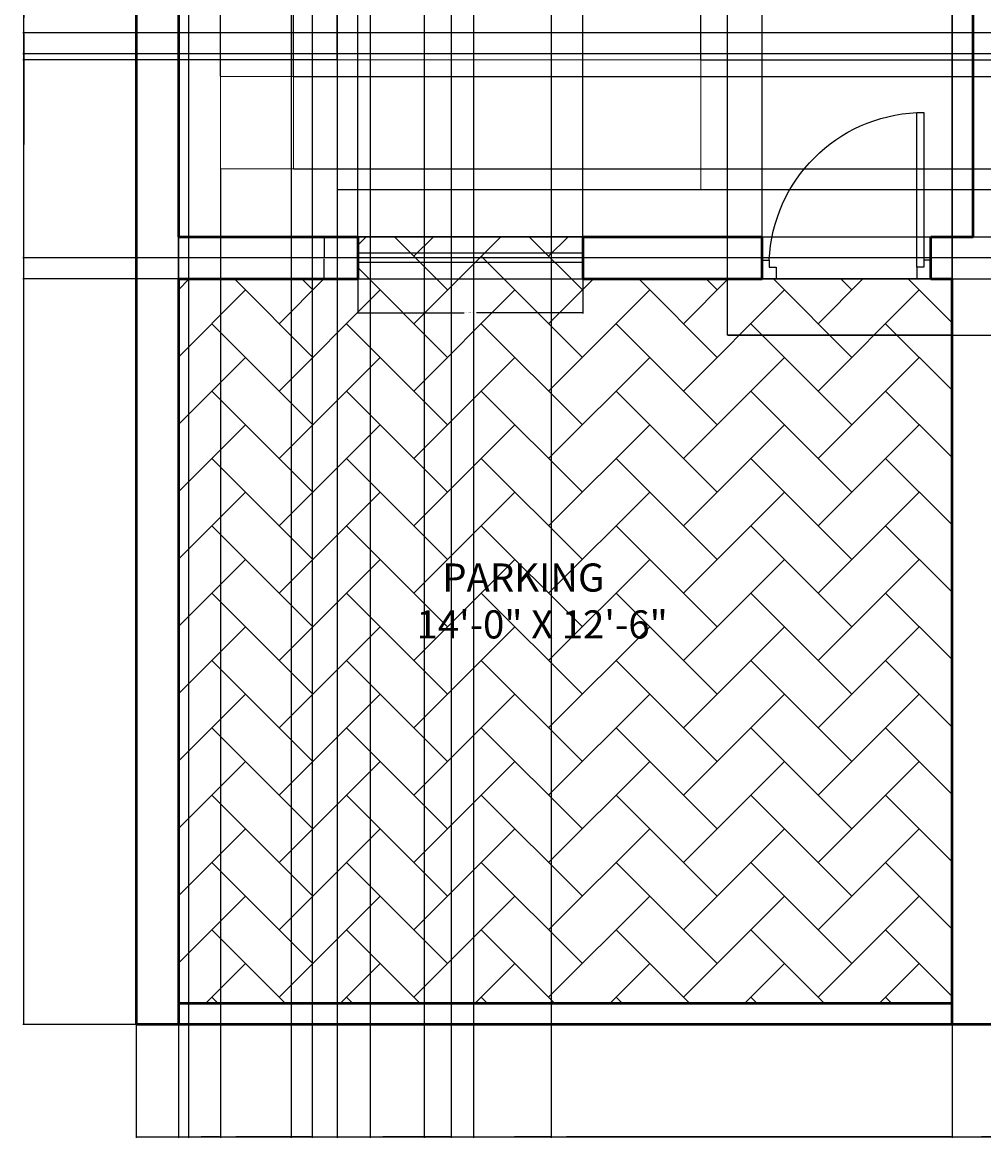
# Model space of a CAD drawing. Units: inches. Extents: x 2330 to 2739, y 947 to 1475.
# Tile 1 of 6: x 2330 to 2535, y 947 to 1185. Entities that reach past the tile are written whole.
import ezdxf

# ---------------------------------------------------------------- set-up
doc = ezdxf.new("R2010")
doc.units = ezdxf.units.IN
for name, color, linetype, lineweight in [('A-ANNO-DIMS', 2, 'Continuous', 18), ('A-AREA-IDEN', 7, 'Continuous', 25), ('A-FLOR-PATT', 252, 'Continuous', 13), ('door', 150, 'Continuous', 25), ('furniture', 9, 'Continuous', 18), ('staircase', 51, 'Continuous', 25), ('wall', 7, 'Continuous', 50), ('window', 40, 'Continuous', 25)]:
    doc.layers.add(name, color=color, linetype=linetype, lineweight=lineweight)
doc.styles.get("Standard").update_dxf_attribs({"font": 'arial.ttf'})
doc.dimstyles.get("Standard").update_dxf_attribs({"dimtxt": 0.18, "dimasz": 0.18, "dimexe": 0.18, "dimexo": 0.0625, "dimgap": 0.09, "dimtad": 0, "dimtih": 1, "dimtoh": 1, "dimdec": 4, "dimzin": 0, "dimdsep": 46, "dimtxsty": 'Standard', "dimcen": 0.09, "dimadec": 0, "dimazin": 0, "dimtfac": 1, "dimtdec": 4, "dimtofl": 0, "dimtmove": 0, "dimatfit": 3, "dimfxl": 1, "dimtolj": 1, "dimtzin": 0, "dimarcsym": 0})

# ---------------------------------------------------------------- blocks, each defined once
blk = doc.blocks.new('w1')
at = {"layer": 'window'}
for p, q in [((2786.57, 1274.71), (2786.57, 1226.71)), ((2788.57, 1274.71), (2788.57, 1226.71))]:
    blk.add_line(p, q, dxfattribs=at)
blk.add_lwpolyline([(2783.07, 1226.71), (2792.07, 1226.71), (2792.07, 1274.71), (2783.07, 1274.71)], close=True, dxfattribs=at)
blk = doc.blocks.new('d1')
at = {"layer": 'door'}
blk.add_line((2897.27, 1313.4), (2933.27, 1313.4), dxfattribs=at)
blk.add_lwpolyline([(2898.77, 1315.9), (2900.27, 1315.9), (2900.27, 1348.9), (2898.77, 1348.9)], close=True, dxfattribs=at)
for points in [[(2900.27, 1313.4), (2897.27, 1313.4), (2897.27, 1317.4), (2898.77, 1317.4), (2898.77, 1315.9), (2900.27, 1315.9), (2900.27, 1313.4)], [(2930.27, 1313.4), (2933.27, 1313.4), (2933.27, 1317.4), (2931.77, 1317.4), (2931.77, 1315.9), (2930.27, 1315.9), (2930.27, 1313.4)]]:
    blk.add_lwpolyline(points, dxfattribs=at)
blk.add_arc((2898.77, 1315.9), 33.03, 2.6026, 87.3974, dxfattribs=at)
blk = doc.blocks.new('*D12')
at = {"layer": 'A-ANNO-DIMS', "color": 0, "lineweight": -2, "transparency": 16777216}
for p, q in [((2401.93, 1130.22), (2401.93, 1122.9)), ((2449.93, 1130.22), (2449.93, 1122.9)), ((2402.11, 1123.08), (2424.59, 1123.08)), ((2449.75, 1123.08), (2427.27, 1123.08))]:
    blk.add_line(p, q, dxfattribs=at)
at = {"layer": 'A-ANNO-DIMS', "color": 0, "transparency": 16777216}
for points in [[(2402.11, 1123.11), (2402.11, 1123.05), (2401.93, 1123.08)], [(2449.75, 1123.11), (2449.75, 1123.05), (2449.93, 1123.08)]]:
    blk.add_solid(points, dxfattribs=at)
at = {"layer": 'Defpoints', "color": 0, "transparency": 16777216}
for p in [(2401.93, 1130.28), (2449.93, 1130.28), (2449.93, 1123.08)]:
    blk.add_point(p, dxfattribs=at)
at = {"layer": 'A-ANNO-DIMS', "color": 0, "transparency": 16777216, "insert": (2425.93, 1123.08), "char_height": 0.18, "attachment_point": 5}
blk.add_mtext('\\A1;WINDOW W1 48 TYP.', dxfattribs=at)
blk = doc.blocks.new('*D13')
at = {"layer": 'A-ANNO-DIMS', "color": 0, "lineweight": -2, "transparency": 16777216}
for p, q in [((2401.87, 1139.28), (2394.55, 1139.28)), ((2394.73, 1139.1), (2394.73, 1134.96)), ((2394.73, 1130.46), (2394.73, 1134.6)), ((2401.87, 1130.28), (2394.55, 1130.28))]:
    blk.add_line(p, q, dxfattribs=at)
at = {"layer": 'A-ANNO-DIMS', "color": 0, "transparency": 16777216}
for points in [[(2394.7, 1139.1), (2394.76, 1139.1), (2394.73, 1139.28)], [(2394.7, 1130.46), (2394.76, 1130.46), (2394.73, 1130.28)]]:
    blk.add_solid(points, dxfattribs=at)
at = {"layer": 'Defpoints', "color": 0, "transparency": 16777216}
for p in [(2401.93, 1139.28), (2394.73, 1130.28), (2401.93, 1130.28)]:
    blk.add_point(p, dxfattribs=at)
at = {"layer": 'A-ANNO-DIMS', "color": 0, "transparency": 16777216, "insert": (2394.73, 1134.78), "char_height": 0.18, "attachment_point": 5}
blk.add_mtext('\\A1;9 TYP.', dxfattribs=at)
blk = doc.blocks.new('*D24')
at = {"layer": 'A-ANNO-DIMS', "color": 0, "lineweight": -2, "transparency": 16777216}
for p, q in [((2354.68, 971.22), (2354.68, 947.1)), ((2714.68, 971.22), (2714.68, 947.1)), ((2354.86, 947.28), (2534.39, 947.28)), ((2714.5, 947.28), (2534.97, 947.28))]:
    blk.add_line(p, q, dxfattribs=at)
at = {"layer": 'A-ANNO-DIMS', "color": 0, "transparency": 16777216}
for points in [[(2354.86, 947.31), (2354.86, 947.25), (2354.68, 947.28)], [(2714.5, 947.31), (2714.5, 947.25), (2714.68, 947.28)]]:
    blk.add_solid(points, dxfattribs=at)
at = {"layer": 'Defpoints', "color": 0, "transparency": 16777216}
for p in [(2354.68, 971.28), (2714.68, 971.28), (2714.68, 947.28)]:
    blk.add_point(p, dxfattribs=at)
at = {"layer": 'A-ANNO-DIMS', "color": 0, "transparency": 16777216, "insert": (2534.68, 947.28), "char_height": 0.18, "attachment_point": 5}
blk.add_mtext('\\A1;360', dxfattribs=at)
blk = doc.blocks.new('*D25')
at = {"layer": 'A-ANNO-DIMS', "color": 0, "lineweight": -2, "transparency": 16777216}
for p, q in [((2354.62, 1451.28), (2330.5, 1451.28)), ((2330.68, 1451.1), (2330.68, 1211.46)), ((2330.68, 971.46), (2330.68, 1211.1)), ((2354.62, 971.28), (2330.5, 971.28))]:
    blk.add_line(p, q, dxfattribs=at)
at = {"layer": 'A-ANNO-DIMS', "color": 0, "transparency": 16777216}
for points in [[(2330.65, 1451.1), (2330.71, 1451.1), (2330.68, 1451.28)], [(2330.65, 971.46), (2330.71, 971.46), (2330.68, 971.28)]]:
    blk.add_solid(points, dxfattribs=at)
at = {"layer": 'Defpoints', "color": 0, "transparency": 16777216}
for p in [(2330.68, 1451.28), (2354.68, 1451.28), (2354.68, 971.28)]:
    blk.add_point(p, dxfattribs=at)
at = {"layer": 'A-ANNO-DIMS', "color": 0, "transparency": 16777216, "insert": (2330.68, 1211.28), "char_height": 0.18, "attachment_point": 5}
blk.add_mtext('\\A1;480', dxfattribs=at)
blk = doc.blocks.new('*D26')
at = {"layer": 'A-ANNO-DIMS', "color": 0, "lineweight": -2, "transparency": 16777216}
for p, q in [((2363.68, 1130.22), (2363.68, 947.1)), ((2528.68, 1130.22), (2528.68, 947.1)), ((2363.86, 947.28), (2445.9, 947.28)), ((2528.5, 947.28), (2446.46, 947.28))]:
    blk.add_line(p, q, dxfattribs=at)
at = {"layer": 'A-ANNO-DIMS', "color": 0, "transparency": 16777216}
for points in [[(2363.86, 947.31), (2363.86, 947.25), (2363.68, 947.28)], [(2528.5, 947.31), (2528.5, 947.25), (2528.68, 947.28)]]:
    blk.add_solid(points, dxfattribs=at)
at = {"layer": 'Defpoints', "color": 0, "transparency": 16777216}
for p in [(2363.68, 1130.28), (2528.68, 1130.28), (2528.68, 947.28)]:
    blk.add_point(p, dxfattribs=at)
at = {"layer": 'A-ANNO-DIMS', "color": 0, "transparency": 16777216, "insert": (2446.18, 947.28), "char_height": 0.18, "attachment_point": 5}
blk.add_mtext('\\A1;165', dxfattribs=at)
blk = doc.blocks.new('*D30')
at = {"layer": 'A-ANNO-DIMS', "color": 0, "lineweight": -2, "transparency": 16777216}
for p, q in [((2677.12, 1182.78), (2330.5, 1182.78)), ((2330.68, 1182.6), (2330.68, 1158.96)), ((2330.68, 1134.96), (2330.68, 1158.6)), ((2677.12, 1134.78), (2330.5, 1134.78))]:
    blk.add_line(p, q, dxfattribs=at)
at = {"layer": 'A-ANNO-DIMS', "color": 0, "transparency": 16777216}
for points in [[(2330.65, 1182.6), (2330.71, 1182.6), (2330.68, 1182.78)], [(2330.65, 1134.96), (2330.71, 1134.96), (2330.68, 1134.78)]]:
    blk.add_solid(points, dxfattribs=at)
at = {"layer": 'Defpoints', "color": 0, "transparency": 16777216}
for p in [(2330.68, 1182.78), (2677.18, 1182.78), (2677.18, 1134.78)]:
    blk.add_point(p, dxfattribs=at)
at = {"layer": 'A-ANNO-DIMS', "color": 0, "transparency": 16777216, "insert": (2330.68, 1158.78), "char_height": 0.18, "attachment_point": 5}
blk.add_mtext('\\A1;48', dxfattribs=at)
blk = doc.blocks.new('*D31')
at = {"layer": 'A-ANNO-DIMS', "color": 0, "lineweight": -2, "transparency": 16777216}
for p, q in [((2363.62, 1317.78), (2330.5, 1317.78)), ((2330.68, 1317.6), (2330.68, 1224.21)), ((2330.68, 1130.46), (2330.68, 1223.85)), ((2363.62, 1130.28), (2330.5, 1130.28))]:
    blk.add_line(p, q, dxfattribs=at)
at = {"layer": 'A-ANNO-DIMS', "color": 0, "transparency": 16777216}
for points in [[(2330.65, 1317.6), (2330.71, 1317.6), (2330.68, 1317.78)], [(2330.65, 1130.46), (2330.71, 1130.46), (2330.68, 1130.28)]]:
    blk.add_solid(points, dxfattribs=at)
at = {"layer": 'Defpoints', "color": 0, "transparency": 16777216}
for p in [(2330.68, 1317.78), (2363.68, 1317.78), (2363.68, 1130.28)]:
    blk.add_point(p, dxfattribs=at)
at = {"layer": 'A-ANNO-DIMS', "color": 0, "transparency": 16777216, "insert": (2330.68, 1224.03), "char_height": 0.18, "attachment_point": 5}
blk.add_mtext('\\A1;187.5', dxfattribs=at)
blk = doc.blocks.new('*D33')
at = {"layer": 'A-ANNO-DIMS', "color": 0, "lineweight": -2, "transparency": 16777216}
for p, q in [((2363.68, 1130.34), (2363.68, 1475.46)), ((2363.86, 1475.28), (2382.41, 1475.28)), ((2401.75, 1475.28), (2383.2, 1475.28)), ((2401.93, 1130.34), (2401.93, 1475.46))]:
    blk.add_line(p, q, dxfattribs=at)
at = {"layer": 'A-ANNO-DIMS', "color": 0, "transparency": 16777216}
for points in [[(2363.86, 1475.31), (2363.86, 1475.25), (2363.68, 1475.28)], [(2401.75, 1475.31), (2401.75, 1475.25), (2401.93, 1475.28)]]:
    blk.add_solid(points, dxfattribs=at)
at = {"layer": 'Defpoints', "color": 0, "transparency": 16777216}
for p in [(2401.93, 1475.28), (2363.68, 1130.28), (2401.93, 1130.28)]:
    blk.add_point(p, dxfattribs=at)
at = {"layer": 'A-ANNO-DIMS', "color": 0, "transparency": 16777216, "insert": (2382.8, 1475.28), "char_height": 0.18, "attachment_point": 5}
blk.add_mtext('\\A1;38.25', dxfattribs=at)
blk = doc.blocks.new('*D34')
at = {"layer": 'A-ANNO-DIMS', "color": 0, "lineweight": -2, "transparency": 16777216}
for p, q in [((2449.93, 1139.34), (2449.93, 1475.46)), ((2450.11, 1475.28), (2468.66, 1475.28)), ((2488, 1475.28), (2469.45, 1475.28)), ((2488.18, 1139.34), (2488.18, 1475.46))]:
    blk.add_line(p, q, dxfattribs=at)
at = {"layer": 'A-ANNO-DIMS', "color": 0, "transparency": 16777216}
for points in [[(2450.11, 1475.31), (2450.11, 1475.25), (2449.93, 1475.28)], [(2488, 1475.31), (2488, 1475.25), (2488.18, 1475.28)]]:
    blk.add_solid(points, dxfattribs=at)
at = {"layer": 'Defpoints', "color": 0, "transparency": 16777216}
for p in [(2488.18, 1475.28), (2449.93, 1139.28), (2488.18, 1139.28)]:
    blk.add_point(p, dxfattribs=at)
at = {"layer": 'A-ANNO-DIMS', "color": 0, "transparency": 16777216, "insert": (2469.05, 1475.28), "char_height": 0.18, "attachment_point": 5}
blk.add_mtext('\\A1;38.25', dxfattribs=at)
blk = doc.blocks.new('*D36')
at = {"layer": 'A-ANNO-DIMS', "color": 0, "lineweight": -2, "transparency": 16777216}
for p, q in [((2528.68, 1394.22), (2528.68, 947.1)), ((2550.43, 1394.22), (2550.43, 947.1)), ((2528.86, 947.28), (2539.16, 947.28)), ((2550.25, 947.28), (2539.95, 947.28))]:
    blk.add_line(p, q, dxfattribs=at)
at = {"layer": 'A-ANNO-DIMS', "color": 0, "transparency": 16777216}
for points in [[(2528.86, 947.31), (2528.86, 947.25), (2528.68, 947.28)], [(2550.25, 947.31), (2550.25, 947.25), (2550.43, 947.28)]]:
    blk.add_solid(points, dxfattribs=at)
at = {"layer": 'Defpoints', "color": 0, "transparency": 16777216}
for p in [(2528.68, 1394.28), (2550.43, 1394.28), (2550.43, 947.28)]:
    blk.add_point(p, dxfattribs=at)
at = {"layer": 'A-ANNO-DIMS', "color": 0, "transparency": 16777216, "insert": (2539.55, 947.28), "char_height": 0.18, "attachment_point": 5}
blk.add_mtext('\\A1;21.75', dxfattribs=at)
blk = doc.blocks.new('*D43')
at = {"layer": 'A-ANNO-DIMS', "color": 0, "lineweight": -2, "transparency": 16777216}
for p, q in [((2593.12, 1182.78), (2330.5, 1182.78)), ((2330.68, 1182.6), (2330.68, 1180.71)), ((2330.68, 1178.46), (2330.68, 1180.35)), ((2593.12, 1178.28), (2330.5, 1178.28))]:
    blk.add_line(p, q, dxfattribs=at)
at = {"layer": 'A-ANNO-DIMS', "color": 0, "transparency": 16777216}
for points in [[(2330.65, 1182.6), (2330.71, 1182.6), (2330.68, 1182.78)], [(2330.65, 1178.46), (2330.71, 1178.46), (2330.68, 1178.28)]]:
    blk.add_solid(points, dxfattribs=at)
at = {"layer": 'Defpoints', "color": 0, "transparency": 16777216}
for p in [(2593.18, 1182.78), (2330.68, 1178.28), (2593.18, 1178.28)]:
    blk.add_point(p, dxfattribs=at)
at = {"layer": 'A-ANNO-DIMS', "color": 0, "transparency": 16777216, "insert": (2330.68, 1180.53), "char_height": 0.18, "attachment_point": 5}
blk.add_mtext('\\A1;4.5', dxfattribs=at)
blk = doc.blocks.new('*D48')
at = {"layer": 'A-ANNO-DIMS', "color": 0, "lineweight": -2, "transparency": 16777216}
for p, q in [((2397.55, 1177.11), (2397.55, 1475.46)), ((2397.73, 1475.28), (2435.93, 1475.28)), ((2474.92, 1475.28), (2436.72, 1475.28)), ((2475.1, 1177.11), (2475.1, 1475.46))]:
    blk.add_line(p, q, dxfattribs=at)
at = {"layer": 'A-ANNO-DIMS', "color": 0, "transparency": 16777216}
for points in [[(2397.73, 1475.31), (2397.73, 1475.25), (2397.55, 1475.28)], [(2474.92, 1475.31), (2474.92, 1475.25), (2475.1, 1475.28)]]:
    blk.add_solid(points, dxfattribs=at)
at = {"layer": 'Defpoints', "color": 0, "transparency": 16777216}
for p in [(2475.1, 1475.28), (2397.55, 1177.05), (2475.1, 1177.05)]:
    blk.add_point(p, dxfattribs=at)
at = {"layer": 'A-ANNO-DIMS', "color": 0, "transparency": 16777216, "insert": (2436.33, 1475.28), "char_height": 0.18, "attachment_point": 5}
blk.add_mtext('\\A1;77.54', dxfattribs=at)
blk = doc.blocks.new('*D49')
at = {"layer": 'A-ANNO-DIMS', "color": 0, "lineweight": -2, "transparency": 16777216}
for p, q in [((2475.16, 1177.05), (2738.86, 1177.05)), ((2738.68, 1176.87), (2738.68, 1163.39)), ((2738.68, 1149.54), (2738.68, 1163.02)), ((2475.16, 1149.36), (2738.86, 1149.36))]:
    blk.add_line(p, q, dxfattribs=at)
at = {"layer": 'A-ANNO-DIMS', "color": 0, "transparency": 16777216}
for points in [[(2738.65, 1176.87), (2738.71, 1176.87), (2738.68, 1177.05)], [(2738.65, 1149.54), (2738.71, 1149.54), (2738.68, 1149.36)]]:
    blk.add_solid(points, dxfattribs=at)
at = {"layer": 'Defpoints', "color": 0, "transparency": 16777216}
for p in [(2475.1, 1177.05), (2475.1, 1149.36), (2738.68, 1149.36)]:
    blk.add_point(p, dxfattribs=at)
at = {"layer": 'A-ANNO-DIMS', "color": 0, "transparency": 16777216, "insert": (2738.68, 1163.21), "char_height": 0.18, "attachment_point": 5}
blk.add_mtext('\\A1;27.687', dxfattribs=at)
blk = doc.blocks.new('*D50')
at = {"layer": 'A-ANNO-DIMS', "color": 0, "lineweight": -2, "transparency": 16777216}
for p, q in [((2372.63, 1173.51), (2372.63, 1475.46)), ((2372.81, 1475.28), (2379.98, 1475.28)), ((2388.05, 1475.28), (2380.88, 1475.28)), ((2388.23, 1173.51), (2388.23, 1475.46))]:
    blk.add_line(p, q, dxfattribs=at)
at = {"layer": 'A-ANNO-DIMS', "color": 0, "transparency": 16777216}
for points in [[(2372.81, 1475.31), (2372.81, 1475.25), (2372.63, 1475.28)], [(2388.05, 1475.31), (2388.05, 1475.25), (2388.23, 1475.28)]]:
    blk.add_solid(points, dxfattribs=at)
at = {"layer": 'Defpoints', "color": 0, "transparency": 16777216}
for p in [(2388.23, 1475.28), (2372.63, 1173.45), (2388.23, 1173.45)]:
    blk.add_point(p, dxfattribs=at)
at = {"layer": 'A-ANNO-DIMS', "color": 0, "transparency": 16777216, "insert": (2380.43, 1475.28), "char_height": 0.18, "attachment_point": 5}
blk.add_mtext('\\A1;15.592', dxfattribs=at)
blk = doc.blocks.new('*D51')
at = {"layer": 'A-ANNO-DIMS', "color": 0, "lineweight": -2, "transparency": 16777216}
for p, q in [((2388.29, 1173.45), (2738.86, 1173.45)), ((2738.68, 1173.27), (2738.68, 1163.81)), ((2738.68, 1153.98), (2738.68, 1163.44)), ((2388.29, 1153.8), (2738.86, 1153.8))]:
    blk.add_line(p, q, dxfattribs=at)
at = {"layer": 'A-ANNO-DIMS', "color": 0, "transparency": 16777216}
for points in [[(2738.65, 1173.27), (2738.71, 1173.27), (2738.68, 1173.45)], [(2738.65, 1153.98), (2738.71, 1153.98), (2738.68, 1153.8)]]:
    blk.add_solid(points, dxfattribs=at)
at = {"layer": 'Defpoints', "color": 0, "transparency": 16777216}
for p in [(2388.23, 1173.45), (2388.23, 1153.8), (2738.68, 1153.8)]:
    blk.add_point(p, dxfattribs=at)
at = {"layer": 'A-ANNO-DIMS', "color": 0, "transparency": 16777216, "insert": (2738.68, 1163.63), "char_height": 0.18, "attachment_point": 5}
blk.add_mtext('\\A1;19.643', dxfattribs=at)
blk = doc.blocks.new('*D52')
at = {"layer": 'A-ANNO-DIMS', "color": 0, "lineweight": -2, "transparency": 16777216}
for p, q in [((2372.63, 1153.74), (2372.63, 947.1)), ((2363.68, 1139.22), (2363.68, 947.1)), ((2363.86, 947.28), (2367.76, 947.28)), ((2372.45, 947.28), (2368.55, 947.28))]:
    blk.add_line(p, q, dxfattribs=at)
at = {"layer": 'A-ANNO-DIMS', "color": 0, "transparency": 16777216}
for points in [[(2363.86, 947.31), (2363.86, 947.25), (2363.68, 947.28)], [(2372.45, 947.31), (2372.45, 947.25), (2372.63, 947.28)]]:
    blk.add_solid(points, dxfattribs=at)
at = {"layer": 'Defpoints', "color": 0, "transparency": 16777216}
for p in [(2372.63, 1153.8), (2363.68, 1139.28), (2372.63, 947.28)]:
    blk.add_point(p, dxfattribs=at)
at = {"layer": 'A-ANNO-DIMS', "color": 0, "transparency": 16777216, "insert": (2368.16, 947.28), "char_height": 0.18, "attachment_point": 5}
blk.add_mtext('\\A1;8.956', dxfattribs=at)
blk = doc.blocks.new('*D53')
at = {"layer": 'A-ANNO-DIMS', "color": 0, "lineweight": -2, "transparency": 16777216}
for p, q in [((2416.07, 1197.91), (2416.07, 947.1)), ((2397.55, 1194.83), (2397.55, 947.1)), ((2397.73, 947.28), (2406.36, 947.28)), ((2415.89, 947.28), (2407.27, 947.28))]:
    blk.add_line(p, q, dxfattribs=at)
at = {"layer": 'A-ANNO-DIMS', "color": 0, "transparency": 16777216}
for points in [[(2397.73, 947.31), (2397.73, 947.25), (2397.55, 947.28)], [(2415.89, 947.31), (2415.89, 947.25), (2416.07, 947.28)]]:
    blk.add_solid(points, dxfattribs=at)
at = {"layer": 'Defpoints', "color": 0, "transparency": 16777216}
for p in [(2416.07, 1197.97), (2397.55, 1194.9), (2416.07, 947.28)]:
    blk.add_point(p, dxfattribs=at)
at = {"layer": 'A-ANNO-DIMS', "color": 0, "transparency": 16777216, "insert": (2406.81, 947.28), "char_height": 0.18, "attachment_point": 5}
blk.add_mtext('\\A1;18.514', dxfattribs=at)
blk = doc.blocks.new('*D54')
at = {"layer": 'A-ANNO-DIMS', "color": 0, "lineweight": -2, "transparency": 16777216}
for p, q in [((2397.49, 1194.9), (2330.5, 1194.9)), ((2330.68, 1194.72), (2330.68, 1186.15)), ((2330.68, 1177.23), (2330.68, 1185.79)), ((2397.49, 1177.05), (2330.5, 1177.05))]:
    blk.add_line(p, q, dxfattribs=at)
at = {"layer": 'A-ANNO-DIMS', "color": 0, "transparency": 16777216}
for points in [[(2330.65, 1194.72), (2330.71, 1194.72), (2330.68, 1194.9)], [(2330.65, 1177.23), (2330.71, 1177.23), (2330.68, 1177.05)]]:
    blk.add_solid(points, dxfattribs=at)
at = {"layer": 'Defpoints', "color": 0, "transparency": 16777216}
for p in [(2330.68, 1194.9), (2397.55, 1194.9), (2397.55, 1177.05)]:
    blk.add_point(p, dxfattribs=at)
at = {"layer": 'A-ANNO-DIMS', "color": 0, "transparency": 16777216, "insert": (2330.68, 1185.97), "char_height": 0.18, "attachment_point": 5}
blk.add_mtext('\\A1;17.85', dxfattribs=at)
blk = doc.blocks.new('*D55')
at = {"layer": 'A-ANNO-DIMS', "color": 0, "lineweight": -2, "transparency": 16777216}
for p, q in [((2397.62, 1149.36), (2738.86, 1149.36)), ((2738.68, 1149.18), (2738.68, 1144.5)), ((2738.68, 1139.46), (2738.68, 1144.14)), ((2401.99, 1139.28), (2738.86, 1139.28))]:
    blk.add_line(p, q, dxfattribs=at)
at = {"layer": 'A-ANNO-DIMS', "color": 0, "transparency": 16777216}
for points in [[(2738.65, 1149.18), (2738.71, 1149.18), (2738.68, 1149.36)], [(2738.65, 1139.46), (2738.71, 1139.46), (2738.68, 1139.28)]]:
    blk.add_solid(points, dxfattribs=at)
at = {"layer": 'Defpoints', "color": 0, "transparency": 16777216}
for p in [(2397.55, 1149.36), (2738.68, 1149.36), (2401.93, 1139.28)]:
    blk.add_point(p, dxfattribs=at)
at = {"layer": 'A-ANNO-DIMS', "color": 0, "transparency": 16777216, "insert": (2738.68, 1144.32), "char_height": 0.18, "attachment_point": 5}
blk.add_mtext('\\A1;10.08', dxfattribs=at)
blk = doc.blocks.new('*D59')
at = {"layer": 'A-ANNO-DIMS', "color": 0, "lineweight": -2, "transparency": 16777216}
for p, q in [((2363.68, 1352.36), (2363.68, 947.1)), ((2387.68, 1352.36), (2387.68, 947.1)), ((2363.86, 947.28), (2375.46, 947.28)), ((2387.5, 947.28), (2375.9, 947.28))]:
    blk.add_line(p, q, dxfattribs=at)
at = {"layer": 'A-ANNO-DIMS', "color": 0, "transparency": 16777216}
for points in [[(2363.86, 947.31), (2363.86, 947.25), (2363.68, 947.28)], [(2387.5, 947.31), (2387.5, 947.25), (2387.68, 947.28)]]:
    blk.add_solid(points, dxfattribs=at)
at = {"layer": 'Defpoints', "color": 0, "transparency": 16777216}
for p in [(2363.68, 1352.42), (2387.68, 1352.42), (2387.68, 947.28)]:
    blk.add_point(p, dxfattribs=at)
at = {"layer": 'A-ANNO-DIMS', "color": 0, "transparency": 16777216, "insert": (2375.68, 947.28), "char_height": 0.18, "attachment_point": 5}
blk.add_mtext('\\A1;24', dxfattribs=at)
blk = doc.blocks.new('*D63')
at = {"layer": 'A-ANNO-DIMS', "color": 0, "lineweight": -2, "transparency": 16777216}
for p, q in [((2426.64, 1421.71), (2426.64, 947.1)), ((2443.2, 1418.22), (2443.2, 947.1)), ((2426.82, 947.28), (2434.46, 947.28)), ((2443.02, 947.28), (2435.37, 947.28))]:
    blk.add_line(p, q, dxfattribs=at)
at = {"layer": 'A-ANNO-DIMS', "color": 0, "transparency": 16777216}
for points in [[(2426.82, 947.31), (2426.82, 947.25), (2426.64, 947.28)], [(2443.02, 947.31), (2443.02, 947.25), (2443.2, 947.28)]]:
    blk.add_solid(points, dxfattribs=at)
at = {"layer": 'Defpoints', "color": 0, "transparency": 16777216}
for p in [(2426.64, 1421.77), (2443.2, 1418.28), (2443.2, 947.28)]:
    blk.add_point(p, dxfattribs=at)
at = {"layer": 'A-ANNO-DIMS', "color": 0, "transparency": 16777216, "insert": (2434.92, 947.28), "char_height": 0.18, "attachment_point": 5}
blk.add_mtext('\\A1;16.556', dxfattribs=at)
blk = doc.blocks.new('*D65')
at = {"layer": 'A-ANNO-DIMS', "color": 0, "lineweight": -2, "transparency": 16777216}
for p, q in [((2404.54, 1425.36), (2404.54, 947.1)), ((2421.84, 1425.36), (2421.84, 947.1)), ((2404.72, 947.28), (2412.73, 947.28)), ((2421.66, 947.28), (2413.64, 947.28))]:
    blk.add_line(p, q, dxfattribs=at)
at = {"layer": 'A-ANNO-DIMS', "color": 0, "transparency": 16777216}
for points in [[(2404.72, 947.31), (2404.72, 947.25), (2404.54, 947.28)], [(2421.66, 947.31), (2421.66, 947.25), (2421.84, 947.28)]]:
    blk.add_solid(points, dxfattribs=at)
at = {"layer": 'Defpoints', "color": 0, "transparency": 16777216}
for p in [(2404.54, 1425.42), (2421.84, 1425.42), (2421.84, 947.28)]:
    blk.add_point(p, dxfattribs=at)
at = {"layer": 'A-ANNO-DIMS', "color": 0, "transparency": 16777216, "insert": (2413.19, 947.28), "char_height": 0.18, "attachment_point": 5}
blk.add_mtext('\\A1;17.295', dxfattribs=at)
blk = doc.blocks.new('*D70')
at = {"layer": 'A-ANNO-DIMS', "color": 0, "lineweight": -2, "transparency": 16777216}
for p, q in [((2365.79, 1325.96), (2365.79, 947.1)), ((2392.19, 1325.96), (2392.19, 947.1)), ((2365.97, 947.28), (2378.67, 947.28)), ((2392.01, 947.28), (2379.32, 947.28))]:
    blk.add_line(p, q, dxfattribs=at)
at = {"layer": 'A-ANNO-DIMS', "color": 0, "transparency": 16777216}
for points in [[(2365.97, 947.31), (2365.97, 947.25), (2365.79, 947.28)], [(2392.01, 947.31), (2392.01, 947.25), (2392.19, 947.28)]]:
    blk.add_solid(points, dxfattribs=at)
at = {"layer": 'Defpoints', "color": 0, "transparency": 16777216}
for p in [(2365.79, 1326.03), (2392.19, 1326.03), (2392.19, 947.28)]:
    blk.add_point(p, dxfattribs=at)
at = {"layer": 'A-ANNO-DIMS', "color": 0, "transparency": 16777216, "insert": (2378.99, 947.28), "char_height": 0.18, "attachment_point": 5}
blk.add_mtext('\\A1;26.4', dxfattribs=at)
blk = doc.blocks.new('*D80')
at = {"layer": 'A-ANNO-DIMS', "color": 0, "lineweight": -2, "transparency": 16777216}
for p, q in [((2480.81, 1118.34), (2480.81, 1475.46)), ((2480.99, 1475.28), (2504.34, 1475.28)), ((2528.5, 1475.28), (2505.14, 1475.28)), ((2528.68, 1118.34), (2528.68, 1475.46))]:
    blk.add_line(p, q, dxfattribs=at)
at = {"layer": 'A-ANNO-DIMS', "color": 0, "transparency": 16777216}
for points in [[(2480.99, 1475.31), (2480.99, 1475.25), (2480.81, 1475.28)], [(2528.5, 1475.31), (2528.5, 1475.25), (2528.68, 1475.28)]]:
    blk.add_solid(points, dxfattribs=at)
at = {"layer": 'Defpoints', "color": 0, "transparency": 16777216}
for p in [(2528.68, 1475.28), (2480.81, 1118.28), (2528.68, 1118.28)]:
    blk.add_point(p, dxfattribs=at)
at = {"layer": 'A-ANNO-DIMS', "color": 0, "transparency": 16777216, "insert": (2504.74, 1475.28), "char_height": 0.18, "attachment_point": 5}
blk.add_mtext('\\A1;47.87', dxfattribs=at)
blk = doc.blocks.new('*D81')
at = {"layer": 'A-ANNO-DIMS', "color": 0, "lineweight": -2, "transparency": 16777216}
for p, q in [((2480.87, 1130.28), (2738.86, 1130.28)), ((2738.68, 1130.1), (2738.68, 1124.46)), ((2738.68, 1118.46), (2738.68, 1124.1)), ((2480.87, 1118.28), (2738.86, 1118.28))]:
    blk.add_line(p, q, dxfattribs=at)
at = {"layer": 'A-ANNO-DIMS', "color": 0, "transparency": 16777216}
for points in [[(2738.65, 1130.1), (2738.71, 1130.1), (2738.68, 1130.28)], [(2738.65, 1118.46), (2738.71, 1118.46), (2738.68, 1118.28)]]:
    blk.add_solid(points, dxfattribs=at)
at = {"layer": 'Defpoints', "color": 0, "transparency": 16777216}
for p in [(2480.81, 1130.28), (2738.68, 1130.28), (2480.81, 1118.28)]:
    blk.add_point(p, dxfattribs=at)
at = {"layer": 'A-ANNO-DIMS', "color": 0, "transparency": 16777216, "insert": (2738.68, 1124.28), "char_height": 0.18, "attachment_point": 5}
blk.add_mtext('\\A1;12', dxfattribs=at)

msp = doc.modelspace()

# ---------------------------------------------------------------- hatches: boundary and pattern name
at = {"layer": 'A-FLOR-PATT'}
h = msp.add_hatch(dxfattribs=at)
h.set_pattern_fill('AR-HBONE', color=256, scale=0.1)
h.paths.add_polyline_path([(2401.9281, 1139.2823), (2401.9281, 1130.2823), (2449.9281, 1130.2823), (2449.9281, 1139.2823)])
edge = h.paths.add_edge_path(flags=17)
edge.add_line((2449.9281, 1135.7823), (2401.9281, 1135.7823))
edge = h.paths.add_edge_path(flags=17)
edge.add_line((2449.9281, 1133.7823), (2401.9281, 1133.7823))
edge = h.paths.add_edge_path()
edge.add_line((2363.6781, 1130.2823), (2363.6781, 971.2823))
edge.add_line((2363.6781, 975.7823), (2528.6781, 975.7823))
edge.add_line((2528.6781, 971.2823), (2528.6781, 1130.2823))
edge.add_line((2449.9281, 1130.2823), (2488.1781, 1130.2823))
edge.add_line((2363.6781, 1130.2823), (2401.9281, 1130.2823))

# ---------------------------------------------------------------- linework, layer by layer
at = {"layer": 'furniture'}
for points in [[(2397.5542, 1177.0487), (2475.0968, 1177.0487), (2475.0968, 1149.3617), (2397.5542, 1149.3617)], [(2388.2258, 1173.4475), (2372.634, 1173.4475), (2372.634, 1153.8045), (2388.2258, 1153.8045)]]:
    msp.add_lwpolyline(points, close=True, dxfattribs=at)
at = {"layer": 'staircase'}
for p, q in [((2528.6781, 1130.2823), (2480.806, 1130.2823)), ((2480.806, 1118.2823), (2480.806, 1130.2823)), ((2528.6781, 1118.2823), (2480.806, 1118.2823))]:
    msp.add_line(p, q, dxfattribs=at)
at = {"layer": 'wall'}
for p, q in [((2354.6781, 1451.2823), (2354.6781, 971.2823)), ((2363.6781, 1317.7823), (2363.6781, 1139.2823)), ((2533.1781, 1139.2823), (2533.1781, 1187.2823)), ((2363.6781, 1139.2823), (2401.9281, 1139.2823)), ((2401.9281, 1139.2823), (2401.9281, 1130.2823)), ((2449.9281, 1139.2823), (2449.9281, 1130.2823)), ((2449.9281, 1139.2823), (2488.1781, 1139.2823)), ((2488.1781, 1130.2823), (2488.1781, 1139.2823)), ((2524.1781, 1130.2823), (2524.1781, 1139.2823)), ((2524.1781, 1139.2823), (2533.1781, 1139.2823)), ((2363.6781, 1130.2823), (2401.9281, 1130.2823)), ((2363.6781, 1130.2823), (2363.6781, 971.2823)), ((2449.9281, 1130.2823), (2488.1781, 1130.2823)), ((2524.1781, 1130.2823), (2528.6781, 1130.2823)), ((2528.6781, 971.2823), (2528.6781, 1130.2823)), ((2363.6781, 975.7823), (2528.6781, 975.7823)), ((2354.6781, 971.2823), (2597.6781, 971.2823))]:
    msp.add_line(p, q, dxfattribs=at)

# ---------------------------------------------------------------- block references
at = {"layer": 'door', "xscale": -1}
msp.add_blockref('d1', (5421.4472, -183.1167), dxfattribs=at)
at = {"layer": 'window', "rotation": 270}
msp.add_blockref('w1', (1175.2195, 3922.3542), dxfattribs=at)

# ---------------------------------------------------------------- texts
at = {"layer": 'A-AREA-IDEN', "insert": (2414.4428, 1069.5937), "char_height": 6, "attachment_point": 1}
msp.add_mtext_dynamic_manual_height_columns('   PARKING\\P14\'-0" X 12\'-6"', width=63.218259, gutter_width=12.5, heights=[0], dxfattribs=at)

# ---------------------------------------------------------------- dimensions: what is measured, and where the dimension line sits
at = {"layer": 'A-ANNO-DIMS'}
for base, p1, p2, override, picture, middle in [((2401.9281, 1475.2843), (2363.6781, 1130.2823), (2401.9281, 1130.2823), {"dimdec": 2, "dimlfac": 1, "dimrnd": 0, "dimzin": 0, "dimdsep": 46, "dimlunit": 2}, '*D33', (2382.8031, 1475.2843)), ((2388.2258, 1475.2843), (2372.634, 1173.4475), (2388.2258, 1173.4475), {"dimdec": 3, "dimlfac": 1, "dimrnd": 0, "dimzin": 0, "dimdsep": 46, "dimlunit": 2}, '*D50', (2380.4299, 1475.2843)), ((2475.0968, 1475.2843), (2397.5542, 1177.0487), (2475.0968, 1177.0487), {"dimdec": 2, "dimlfac": 1, "dimrnd": 0, "dimzin": 0, "dimdsep": 46, "dimlunit": 2}, '*D48', (2436.3255, 1475.2843)), ((2488.1781, 1475.2843), (2449.9281, 1139.2823), (2488.1781, 1139.2823), {"dimdec": 2, "dimlfac": 1, "dimrnd": 0, "dimzin": 0, "dimdsep": 46, "dimlunit": 2}, '*D34', (2469.0531, 1475.2843)), ((2528.6781, 1475.2843), (2480.806, 1118.2823), (2528.6781, 1118.2823), {"dimdec": 2, "dimlfac": 1, "dimrnd": 0, "dimzin": 0, "dimdsep": 46, "dimlunit": 2}, '*D80', (2504.7421, 1475.2843)), ((2421.8362, 947.2803), (2404.5411, 1425.4192), (2421.8362, 1425.4192), {"dimdec": 3, "dimlfac": 1, "dimrnd": 0, "dimzin": 0, "dimdsep": 46, "dimlunit": 2}, '*D65', (2413.1887, 947.2803)), ((2443.1961, 947.2803), (2426.6405, 1421.7694), (2443.1961, 1418.2823), {"dimdec": 3, "dimlfac": 1, "dimrnd": 0, "dimzin": 0, "dimdsep": 46, "dimlunit": 2}, '*D63', (2434.9183, 947.2803)), ((2550.4281, 947.2803), (2528.6781, 1394.2823), (2550.4281, 1394.2823), {"dimdec": 2, "dimlfac": 1, "dimrnd": 0, "dimzin": 0, "dimdsep": 46, "dimlunit": 2}, '*D36', (2539.5531, 947.2803)), ((2387.6781, 947.2803), (2363.6781, 1352.4216), (2387.6781, 1352.4216), {"dimdec": 0, "dimlfac": 1, "dimrnd": 0, "dimzin": 0, "dimdsep": 46, "dimlunit": 2}, '*D59', (2375.6781, 947.2803)), ((2392.1947, 947.2803), (2365.7931, 1326.0264), (2392.1947, 1326.0264), {"dimdec": 1, "dimlfac": 1, "dimrnd": 0, "dimzin": 0, "dimdsep": 46, "dimlunit": 2}, '*D70', (2378.9939, 947.2803)), ((2416.0685, 947.2803), (2397.5542, 1194.8972), (2416.0685, 1197.968), {"dimdec": 3, "dimlfac": 1, "dimrnd": 0, "dimzin": 0, "dimdsep": 46, "dimlunit": 2}, '*D53', (2406.8113, 947.2803)), ((2372.634, 947.2803), (2363.6781, 1139.2823), (2372.634, 1153.8045), {"dimdec": 3, "dimlfac": 1, "dimrnd": 0, "dimzin": 0, "dimdsep": 46, "dimlunit": 2}, '*D52', (2368.156, 947.2803)), ((2528.6781, 947.2803), (2363.6781, 1130.2823), (2528.6781, 1130.2823), {"dimdec": 0, "dimlfac": 1, "dimrnd": 0, "dimzin": 0, "dimdsep": 46, "dimlunit": 2}, '*D26', (2446.1781, 947.2803)), ((2714.6781, 947.2803), (2354.6781, 971.2823), (2714.6781, 971.2823), {"dimdec": 0, "dimlfac": 1, "dimrnd": 0, "dimzin": 0, "dimdsep": 46, "dimlunit": 2}, '*D24', (2534.6781, 947.2803))]:
    dim = msp.add_linear_dim(base=base, p1=p1, p2=p2, dimstyle='Standard', override=override, dxfattribs=at)
    dim.commit()
    dim.dimension.update_dxf_attribs({"geometry": picture, "text_midpoint": middle})
for base, p1, p2, override, picture, middle in [((2330.6761, 1451.2823), (2354.6781, 971.2823), (2354.6781, 1451.2823), {"dimdec": 0, "dimlfac": 1, "dimrnd": 0, "dimzin": 0, "dimdsep": 46, "dimlunit": 2}, '*D25', (2330.6761, 1211.2823)), ((2330.6761, 1317.7823), (2363.6781, 1130.2823), (2363.6781, 1317.7823), {"dimdec": 1, "dimlfac": 1, "dimrnd": 0, "dimzin": 0, "dimdsep": 46, "dimlunit": 2}, '*D31', (2330.6761, 1224.0323)), ((2330.6761, 1194.8972), (2397.5542, 1177.0487), (2397.5542, 1194.8972), {"dimdec": 2, "dimlfac": 1, "dimrnd": 0, "dimzin": 0, "dimdsep": 46, "dimlunit": 2}, '*D54', (2330.6761, 1185.9729)), ((2330.6761, 1182.7823), (2677.1781, 1134.7823), (2677.1781, 1182.7823), {"dimdec": 0, "dimlfac": 1, "dimrnd": 0, "dimzin": 0, "dimdsep": 46, "dimlunit": 2}, '*D30', (2330.6761, 1158.7823)), ((2330.6761, 1178.2823), (2593.1781, 1182.7823), (2593.1781, 1178.2823), {"dimdec": 1, "dimlfac": 1, "dimrnd": 0, "dimzin": 0, "dimdsep": 46, "dimlunit": 2}, '*D43', (2330.6761, 1180.5323)), ((2738.6801, 1149.3617), (2475.0968, 1177.0487), (2475.0968, 1149.3617), {"dimdec": 3, "dimlfac": 1, "dimrnd": 0, "dimzin": 0, "dimdsep": 46, "dimlunit": 2}, '*D49', (2738.6801, 1163.2052)), ((2738.6801, 1153.8045), (2388.2258, 1173.4475), (2388.2258, 1153.8045), {"dimdec": 3, "dimlfac": 1, "dimrnd": 0, "dimzin": 0, "dimdsep": 46, "dimlunit": 2}, '*D51', (2738.6801, 1163.626)), ((2738.6801, 1149.3617), (2401.9281, 1139.2823), (2397.5542, 1149.3617), {"dimdec": 2, "dimlfac": 1, "dimrnd": 0, "dimzin": 0, "dimdsep": 46, "dimlunit": 2}, '*D55', (2738.6801, 1144.322)), ((2738.6801, 1130.2823), (2480.806, 1118.2823), (2480.806, 1130.2823), {"dimdec": 0, "dimlfac": 1, "dimrnd": 0, "dimzin": 0, "dimdsep": 46, "dimlunit": 2}, '*D81', (2738.6801, 1124.2823))]:
    dim = msp.add_linear_dim(base=base, p1=p1, p2=p2, angle=90, dimstyle='Standard', override=override, dxfattribs=at)
    dim.commit()
    dim.dimension.update_dxf_attribs({"geometry": picture, "text_midpoint": middle})
dim = msp.add_linear_dim(base=(2394.7281, 1130.2823), p1=(2401.9281, 1139.2823), p2=(2401.9281, 1130.2823), angle=270, text='<> TYP.', dimstyle='Standard', override={"dimdec": 0, "dimlfac": 1, "dimrnd": 0, "dimzin": 0, "dimdsep": 46, "dimlunit": 2}, dxfattribs=at)
dim.commit()
dim.dimension.update_dxf_attribs({"geometry": '*D13', "text_midpoint": (2394.7281, 1134.7823)})
dim = msp.add_linear_dim(base=(2449.9281, 1123.0823), p1=(2401.9281, 1130.2823), p2=(2449.9281, 1130.2823), text='WINDOW W1 <> TYP.', dimstyle='Standard', override={"dimdec": 0, "dimlfac": 1, "dimrnd": 0, "dimzin": 0, "dimdsep": 46, "dimlunit": 2}, dxfattribs=at)
dim.commit()
dim.dimension.update_dxf_attribs({"geometry": '*D12', "text_midpoint": (2425.9281, 1123.0823)})

doc.saveas('drawing.dxf')
